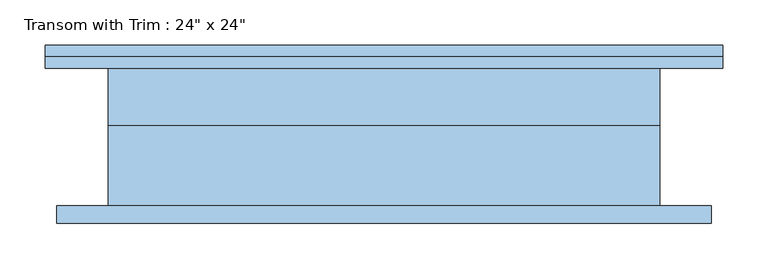
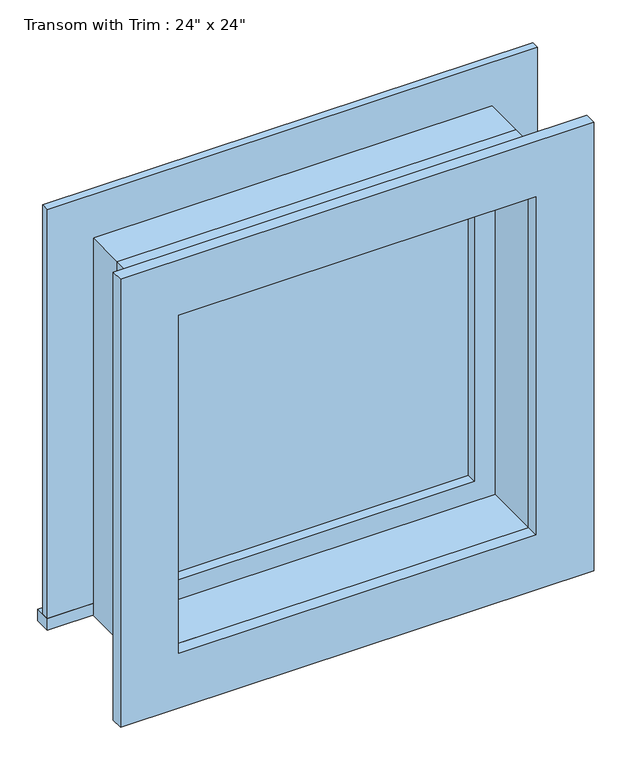
"""IFC4 building model written with IfcOpenShell, lengths in millimetres: window geometry."""

from ifc_helpers import new_model, si_unit, frame, origin, place, context, project, spatial, polyline, outline, extrude, source, transform, mapped, element, save


def window_3d781103(model_context):
    return source(origin(), model_context, "Body", "SweptSolid", [
        extrude(outline(polyline([(-412.75, 101.6), (336.55, 101.6), (336.55, 76.2), (-412.75, 76.2), (-412.75, 101.6)])), frame((0.0, 0.0, 2159.0), z_axis=(0.0, 0.0, 1.0), x_axis=(1.0, 0.0, 0.0)), (0.0, 0.0, 1.0), 19.05),
        extrude(outline(polyline([(2749.55, -323.85), (2749.55, 247.65), (2178.05, 247.65), (2178.05, 336.55), (2838.45, 336.55), (2838.45, -412.75), (2178.05, -412.75), (2178.05, -323.85), (2749.55, -323.85)])), frame((0.0, 76.2, 0.0), z_axis=(0.0, 1.0, 0.0), x_axis=(0.0, 0.0, 1.0)), (0.0, 0.0, 1.0), 12.7),
        extrude(outline(polyline([(2825.75, 323.85), (2825.75, -400.05), (2101.85, -400.05), (2101.85, 323.85), (2825.75, 323.85)]), holes=[polyline([(2736.85, 234.95), (2190.75, 234.95), (2190.75, -311.15), (2736.85, -311.15), (2736.85, 234.95)])]), frame((0.0, -95.25, 0.0), z_axis=(0.0, 1.0, 0.0), x_axis=(0.0, 0.0, 1.0)), (0.0, 0.0, 1.0), 19.05),
        extrude(outline(polyline([(203.2, 28.575), (-279.4, 28.575), (-279.4, 41.275), (203.2, 41.275), (203.2, 28.575)])), frame((0.0, 0.0, 2222.5), z_axis=(0.0, 0.0, 1.0), x_axis=(1.0, 0.0, 0.0)), (0.0, 0.0, 1.0), 482.6),
        extrude(outline(polyline([(2749.55, -323.85), (2178.05, -323.85), (2178.05, 247.65), (2749.55, 247.65), (2749.55, -323.85)]), holes=[polyline([(2705.1, -279.4), (2705.1, 203.2), (2222.5, 203.2), (2222.5, -279.4), (2705.1, -279.4)])]), frame((0.0, 12.7, 0.0), z_axis=(0.0, 1.0, 0.0), x_axis=(0.0, 0.0, 1.0)), (0.0, 0.0, 1.0), 44.45),
        extrude(outline(polyline([(2768.6, -342.9), (2159.0, -342.9), (2159.0, 266.7), (2768.6, 266.7), (2768.6, -342.9)]), holes=[polyline([(2736.85, -311.15), (2736.85, 234.95), (2190.75, 234.95), (2190.75, -311.15), (2736.85, -311.15)])]), frame((0.0, -76.2, 0.0), z_axis=(0.0, 1.0, 0.0), x_axis=(0.0, 0.0, 1.0)), (0.0, 0.0, 1.0), 88.9),
        extrude(outline(polyline([(2768.6, 266.7), (2768.6, -342.9), (2159.0, -342.9), (2159.0, 266.7), (2768.6, 266.7)]), holes=[polyline([(2749.55, 247.65), (2178.05, 247.65), (2178.05, -323.85), (2749.55, -323.85), (2749.55, 247.65)])]), frame((0.0, 12.7, 0.0), z_axis=(0.0, 1.0, 0.0), x_axis=(0.0, 0.0, 1.0)), (0.0, 0.0, 1.0), 63.5),
    ])


if __name__ == "__main__":
    model = new_model("IFC4")
    model_context = context("Model", 3, world=origin())
    ifc_project = project(units=[si_unit("LENGTHUNIT", "METRE", prefix="MILLI")], contexts=[model_context])
    site = spatial("IfcSite", under=ifc_project)
    building = spatial("IfcBuilding", under=site)
    placement = place(None, origin())
    window_shape = window_3d781103(model_context)
    element("IfcWindow", 1, ObjectType="Transom with Trim : 24\" x 24\"", at=placement, inside=building, context=model_context, shape_type="MappedRepresentation", body=[
        mapped(window_shape, transform((0.0, 0.0, 0.0), x_axis=(1.0, 0.0, 0.0), y_axis=(0.0, 1.0, 0.0), z_axis=(0.0, 0.0, 1.0))),
    ])
    save(model, "model.ifc")

# Revit data of these elements
# Type "Transom with Trim : 24\" x 24\""
#   Type Mark = "13"
#   Construction Type Id = "GSP4R"
#   Assembly Code = "B2020100"
#   Analytic Construction = "1/8 in Pilkington single glazing"
#   Visual Light Transmittance = 0.9
#   Solar Heat Gain Coefficient = 0.78
#   Heat Transfer Coefficient (U) = 0.6496 BTU/(h·ft²·°F)
#   Height = 2' - 0"
#   Default Sill Height = 7' - 1"
#   Trim Projection - Ext. = 0' - 0 1/2"
#   Trim Projection - Int. = 0' - 0 3/4"
#   Trim Width - Exterior = 0' - 3 1/2"
#   Trim Width - Interior = 0' - 3 1/2"
#   Width = 2' - 0"
#   Window Inset = 0' - 0 3/4"
#   Define Thermal Properties by = 1
#   Glass Pane Material = Glass
#   Sash Material = Sash
#   Trim Exterior Material = Trim
#   Trim Interior Material = Trim
#   Wall Closure = (empty or 0)
# Element 1 (IfcWindow, "Transom with Trim : 24\" x 24\"")
#   Materials on its faces: "Sash", "Trim", "Glass"
# Materials
#   "Glass": class "Glass", colour RGB 0 128 192, transparency 0.75, Description = "Soda Lime Glass", Cost = 0
#   "Sash": class "Wood", colour RGB 224 178 126, transparency 0
#   "Trim": class "Wood", colour RGB 224 178 126, transparency 0
